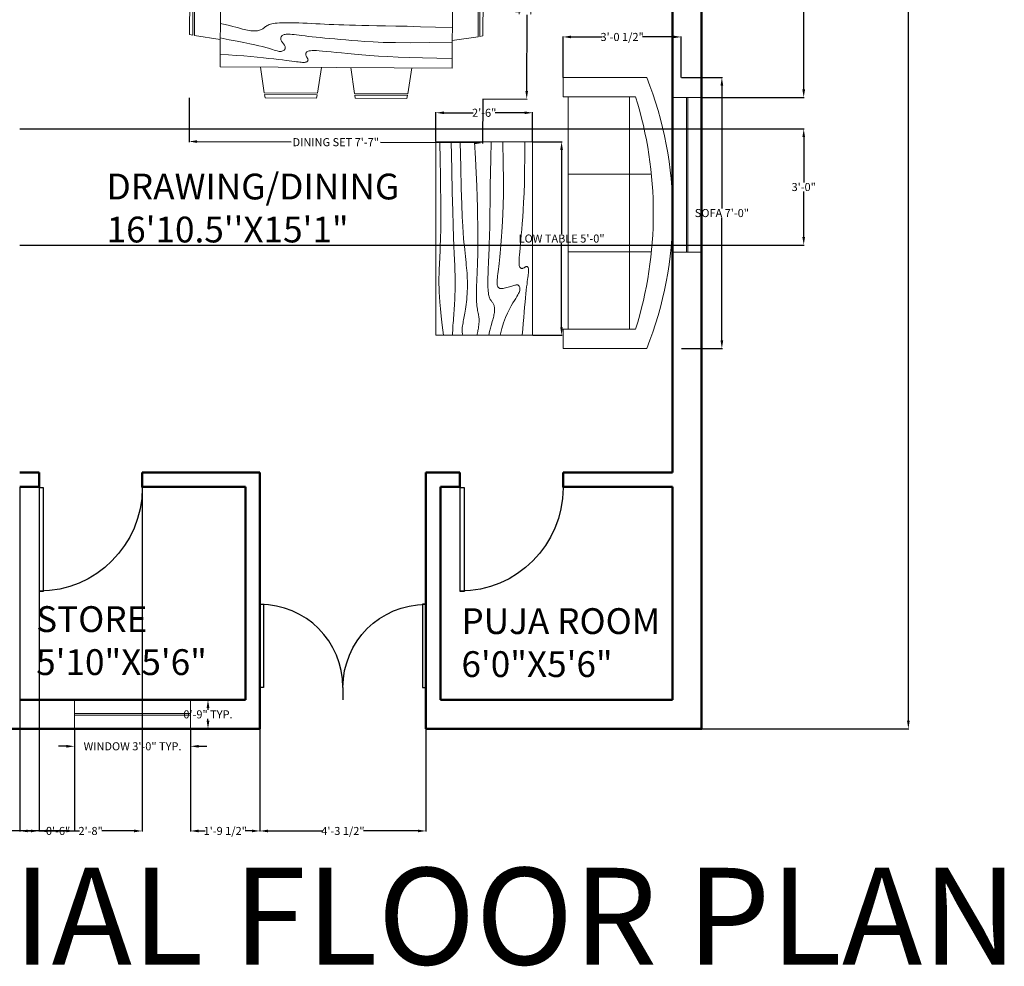
# Model space of a CAD drawing. Units: inches. Extents: x 14 to 510, y 5 to 635.
# Tile 2 of 3: x 205 to 510, y 5 to 299. Entities that reach past the tile are written whole.
import ezdxf

# ---------------------------------------------------------------- set-up
doc = ezdxf.new("R2010")
doc.units = ezdxf.units.IN
doc.header["$MEASUREMENT"] = 0
for name, color, linetype, lineweight in [('A-ANNO-DIMS', 210, 'Continuous', 18), ('A-AREA-IDEN', 210, 'Continuous', 25), ('A-FURN', 100, 'Continuous', 18), ('DOOR', 20, 'Continuous', 25), ('TEXT', 210, 'Continuous', 35), ('WALL', 40, 'Continuous', 50), ('WINDOW', 131, 'Continuous', 18)]:
    doc.layers.add(name, color=color, linetype=linetype, lineweight=lineweight)
doc.styles.get("Standard").update_dxf_attribs({"font": 'arial.ttf'})
doc.dimstyles.get("Standard").update_dxf_attribs({"dimtxt": 2.5, "dimasz": 2.5, "dimexe": 0.18, "dimexo": 0.0625, "dimgap": 0.09, "dimtad": 0, "dimtih": 1, "dimtoh": 1, "dimzin": 0, "dimdsep": 46, "dimlunit": 3, "dimtxsty": 'Standard', "dimcen": 0.09, "dimadec": 0, "dimazin": 0, "dimtfac": 1, "dimtofl": 0, "dimtmove": 0, "dimatfit": 3, "dimfxl": 1, "dimtolj": 1, "dimtzin": 0, "dimarcsym": 0})

# ---------------------------------------------------------------- blocks, each defined once
blk = doc.blocks.new('*U2')
for p, q in [((0, 0), (0, -6)), ((40, 0), (40, -6))]:
    blk.add_line(p, q)
blk.add_lwpolyline([(0, 0), (0, 40), (1.75, 40), (1.75, 0)], close=True)
blk.add_arc((0, 0), 40, 0, 90)
blk = doc.blocks.new('Dining Set - 36 x 72 in.')
for p, q in [((-22, 27.5), (-22.1562, 26.50042)), ((-22, 27.5), (-6, 27.5)), ((-5.8437, 26.49966), (-6, 27.5)), ((6, 27.5), (5.8438, 26.50042)), ((6, 27.5), (22, 27.5)), ((22.1563, 26.49966), (22, 27.5)), ((-22.2343, 26.00059), (-23.4847, 17.99762)), ((-22.2304, 26), (-5.7608, 26)), ((-5.8416, 26.5), (-22.1534, 26.5)), ((-4.5152, 17.99762), (-5.7655, 25.99926)), ((5.7657, 26.00059), (4.5153, 17.99762)), ((5.7696, 26), (22.2392, 26)), ((22.1584, 26.5), (5.8466, 26.5)), ((23.4848, 17.99762), (22.2345, 25.99926)), ((36, 18), (-36, 18)), ((-36, 18), (-36, -18)), ((36, -18), (36, 18)), ((-44.0006, 8.23428), (-35.9976, 9.48474)), ((44.0006, 8.23428), (35.9976, 9.48474)), ((-45.5, 8), (-44.5004, 8.15617)), ((-45.5, 8), (-45.5, -8)), ((-44.5, -8.15843), (-44.5, 8.15338)), ((-44, 8.23041), (-44, -8.23915)), ((44, 8.23041), (44, -8.23915)), ((44.5, -8.15843), (44.5, 8.15338)), ((45.5, 8), (44.5005, 8.15617)), ((45.5, 8), (45.5, -8)), ((-44.4997, -8.15631), (-45.5, -8)), ((-35.9976, -9.48476), (-43.9993, -8.2345)), ((35.9976, -9.48476), (43.9993, -8.2345)), ((44.4997, -8.15631), (45.5, -8)), ((-36, -18), (36, -18)), ((-22.2343, -26.0006), (-23.4847, -17.99762)), ((-4.5152, -17.99762), (-5.7655, -25.99928)), ((5.7657, -26.0006), (4.5153, -17.99762)), ((23.4848, -17.99762), (22.2345, -25.99928)), ((-22.2304, -26), (-5.7608, -26)), ((-22, -27.5), (-22.1562, -26.50044)), ((-5.8416, -26.5), (-22.1534, -26.5)), ((-5.8437, -26.49967), (-6, -27.5)), ((5.7696, -26), (22.2392, -26)), ((6, -27.5), (5.8438, -26.50044)), ((22.1584, -26.5), (5.8466, -26.5)), ((22.1563, -26.49967), (22, -27.5)), ((-22, -27.5), (-6, -27.5)), ((6, -27.5), (22, -27.5))]:
    blk.add_line(p, q)
for points in [[(-36, 15), (-31.1772, 14.97754), (-26.8079, 14.91406), (-22.8538, 14.81543), (-19.276, 14.6875), (-16.0362, 14.53613), (-13.0957, 14.36718), (-10.4159, 14.18652), (-7.9583, 14), (-5.6904, 13.81315), (-3.6035, 13.63021), (-1.6954, 13.45508), (0.0365, 13.29166), (1.5945, 13.14388), (2.9811, 13.01562), (4.1988, 12.9108), (5.25, 12.83333), (6.1393, 12.78613), (6.8802, 12.76823), (7.4883, 12.77767), (7.9792, 12.8125), (8.3685, 12.87077), (8.6719, 12.95052), (8.9049, 13.0498), (9.0833, 13.16666), (9.2205, 13.29899), (9.3216, 13.44401), (9.3895, 13.59879), (9.4271, 13.76041), (9.4373, 13.92594), (9.4232, 14.09245), (9.3875, 14.257), (9.3333, 14.41666), (9.2638, 14.56917), (9.1836, 14.71484), (9.0975, 14.85465), (9.0104, 14.98958), (8.9272, 15.1206), (8.8529, 15.2487), (8.7922, 15.37483), (8.75, 15.5), (8.7305, 15.62467), (8.7344, 15.74739), (8.7617, 15.86621), (8.8125, 15.97916), (8.8867, 16.08431), (8.9844, 16.17968), (9.1055, 16.26334), (9.25, 16.33333), (9.4189, 16.38802), (9.6172, 16.42708), (9.8506, 16.45052), (10.125, 16.45833), (10.4463, 16.45052), (10.8203, 16.42708), (11.2529, 16.38802), (11.75, 16.33333), (12.3184, 16.26318), (12.9694, 16.17838), (13.7151, 16.07991), (14.5677, 15.96875), (15.5395, 15.84586), (16.6426, 15.71224), (17.8893, 15.56884), (19.2917, 15.41666), (20.859, 15.25667), (22.5879, 15.08984), (24.4721, 14.91715), (26.5052, 14.73958), (28.6809, 14.5581), (30.9929, 14.3737), (33.4347, 14.18733), (36, 14)], [(-36, 10), (-28.9766, 10.14274), (-23.1725, 10.20442), (-18.4241, 10.19775), (-14.5677, 10.13541), (-11.4399, 10.03011), (-8.877, 9.89453), (-6.7154, 9.74137), (-4.7917, 9.58333), (-2.9698, 9.43082), (-1.2246, 9.28515), (0.4415, 9.14534), (2.026, 9.01041), (3.5266, 8.87939), (4.9408, 8.7513), (6.266, 8.62516), (7.5, 8.5), (8.6411, 8.37549), (9.6914, 8.2539), (10.6538, 8.13818), (11.5312, 8.03125), (12.3267, 7.93603), (13.043, 7.85547), (13.6831, 7.79248), (14.25, 7.75), (14.7471, 7.7303), (15.1797, 7.73307), (15.5537, 7.75732), (15.875, 7.80208), (16.1494, 7.86637), (16.3828, 7.94922), (16.5811, 8.04964), (16.75, 8.16666), (16.8944, 8.29915), (17.0143, 8.44531), (17.1089, 8.60319), (17.1771, 8.77083), (17.218, 8.94629), (17.2305, 9.1276), (17.2137, 9.31282), (17.1667, 9.5), (17.0895, 9.6875), (16.987, 9.875), (16.8649, 10.0625), (16.7292, 10.25), (16.5856, 10.4375), (16.4401, 10.625), (16.2985, 10.8125), (16.1667, 11), (16.05, 11.18733), (15.9518, 11.3737), (15.8752, 11.5581), (15.8229, 11.73958), (15.798, 11.91715), (15.8034, 12.08984), (15.842, 12.25667), (15.9167, 12.41666), (16.0295, 12.56836), (16.1784, 12.70833), (16.3605, 12.83268), (16.5729, 12.9375), (16.8127, 13.01888), (17.0768, 13.07291), (17.3625, 13.0957), (17.6667, 13.08333), (17.9894, 13.03312), (18.3418, 12.94726), (18.7382, 12.82918), (19.1927, 12.68229), (19.7195, 12.51001), (20.3327, 12.31575), (21.0465, 12.10294), (21.875, 11.875), (22.8357, 11.63354), (23.959, 11.37304), (25.2786, 11.08618), (26.8282, 10.76562), (28.6414, 10.40405), (30.752, 9.99414), (33.1936, 9.52856), (36, 9)], [(-36, 5.5), (-30.7157, 5.3348), (-26.069, 5.20963), (-21.9946, 5.11767), (-18.4271, 5.05208), (-15.3009, 5.00602), (-12.5508, 4.97265), (-10.1112, 4.94515), (-7.9167, 4.91666), (-5.909, 4.88167), (-4.0586, 4.83984), (-2.3429, 4.79215), (-0.7396, 4.73958), (0.7739, 4.6831), (2.22, 4.6237), (3.6213, 4.56233), (5, 4.5), (6.373, 4.43782), (7.7344, 4.3776), (9.0723, 4.32129), (10.375, 4.27083), (11.6309, 4.22819), (12.8281, 4.19531), (13.9551, 4.17415), (15, 4.16666), (15.954, 4.17448), (16.819, 4.19791), (17.6001, 4.23698), (18.3021, 4.29166), (18.9299, 4.36198), (19.4883, 4.44791), (19.9823, 4.54948), (20.4167, 4.66666), (20.7969, 4.79899), (21.1302, 4.94401), (21.4245, 5.09879), (21.6875, 5.26041), (21.9271, 5.42594), (22.1511, 5.59245), (22.3672, 5.757), (22.5834, 5.91666), (22.8065, 6.06868), (23.0404, 6.21093), (23.2879, 6.34147), (23.5521, 6.45833), (23.8358, 6.55957), (24.142, 6.64323), (24.4735, 6.70735), (24.8334, 6.75), (25.2235, 6.76969), (25.642, 6.76692), (26.0858, 6.74267), (26.5521, 6.69791), (27.0379, 6.63362), (27.5404, 6.55078), (28.0565, 6.45036), (28.5834, 6.33333), (29.1242, 6.19987), (29.7071, 6.04687), (30.3661, 5.87044), (31.1354, 5.66666), (32.0493, 5.43164), (33.142, 5.16146), (34.4475, 4.85221), (36, 4.5)], [(-36, -1), (-30.7915, -0.6591), (-26.0195, -0.38216), (-21.6519, -0.16284), (-17.6563, 0.00521), (-14.0005, 0.12833), (-10.6523, 0.21289), (-7.5796, 0.26522), (-4.75, 0.29166), (-2.134, 0.29793), (0.2878, 0.28711), (2.5317, 0.26163), (4.6146, 0.22396), (6.5529, 0.17651), (8.3633, 0.12174), (10.0623, 0.06209), (11.6667, 0), (13.1899, -0.06201), (14.6341, -0.1211), (15.9982, -0.17432), (17.2813, -0.21875), (18.4823, -0.25147), (19.6003, -0.26953), (20.6343, -0.27002), (21.5834, -0.25), (22.4481, -0.20768), (23.2357, -0.14584), (23.9549, -0.06836), (24.6146, 0.02083), (25.2235, 0.11784), (25.7904, 0.21875), (26.3241, 0.31966), (26.8334, 0.41666), (27.3265, 0.50618), (27.8099, 0.58593), (28.2894, 0.65397), (28.7709, 0.70833), (29.2601, 0.74707), (29.763, 0.76823), (30.2855, 0.76985), (30.8334, 0.75), (31.4088, 0.70784), (31.9994, 0.64713), (32.589, 0.57275), (33.1615, 0.48958), (33.7008, 0.4025), (34.1908, 0.3164), (34.6153, 0.23616), (34.9584, 0.16666), (35.2099, 0.11165), (35.3848, 0.07031), (35.504, 0.04069), (35.5886, 0.02083), (35.6594, 0.00879), (35.7377, 0.0026), (35.8442, 0.00032), (36, 0)], [(-36, -6.5), (-27.1843, -6.31267), (-20.084, -6.1263), (-14.469, -5.9419), (-10.1094, -5.76042), (-6.7752, -5.58285), (-4.2363, -5.41016), (-2.2629, -5.24333), (-0.625, -5.08334), (0.8708, -4.93099), (2.2715, -4.78646), (3.5872, -4.64974), (4.8281, -4.52084), (6.0046, -4.39974), (7.127, -4.28646), (8.2053, -4.18099), (9.25, -4.08334), (10.2705, -3.99382), (11.2734, -3.91407), (12.2647, -3.84603), (13.25, -3.79167), (14.2354, -3.75293), (15.2266, -3.73177), (16.2295, -3.73015), (17.25, -3.75), (18.2912, -3.79248), (19.3451, -3.85547), (20.4009, -3.93604), (21.4479, -4.03125), (22.4754, -4.13819), (23.4727, -4.25391), (24.4289, -4.37549), (25.3334, -4.5), (26.1785, -4.62492), (26.9694, -4.74935), (27.7145, -4.87281), (28.4219, -4.99479), (29.1, -5.11483), (29.7572, -5.23242), (30.4016, -5.34709), (31.0417, -5.45834), (31.6837, -5.56437), (32.3262, -5.65821), (32.9658, -5.73153), (33.599, -5.77604), (34.2224, -5.78345), (34.8327, -5.74545), (35.4264, -5.65373), (36, -5.5)], [(-36, -10), (-26.4022, -9.81299), (-18.4675, -9.62891), (-11.9839, -9.45069), (-6.7396, -9.28125), (-2.5226, -9.12354), (0.8789, -8.98047), (3.6769, -8.85498), (6.0833, -8.75), (8.2767, -8.66765), (10.3021, -8.60677), (12.1712, -8.56543), (13.8958, -8.54167), (15.4876, -8.53353), (16.9583, -8.53907), (18.3197, -8.55632), (19.5834, -8.58334), (20.7616, -8.61841), (21.8685, -8.66081), (22.9188, -8.71004), (23.9271, -8.76563), (24.9081, -8.82707), (25.8763, -8.89388), (26.8465, -8.96558), (27.8334, -9.04167), (28.8474, -9.12118), (29.8828, -9.20117), (30.93, -9.27824), (31.9792, -9.34896), (33.0205, -9.40991), (34.0443, -9.45768), (35.0407, -9.48885), (36, -9.5)], [(-36, -14.5), (-30.0881, -14.33513), (-25.0332, -14.21224), (-20.7312, -14.12647), (-17.0781, -14.07292), (-13.97, -14.04671), (-11.3027, -14.04297), (-8.9724, -14.05681), (-6.875, -14.08334), (-4.9224, -14.11833), (-3.0905, -14.16016), (-1.3709, -14.20785), (0.2448, -14.26042), (1.7647, -14.3169), (3.1973, -14.3763), (4.5507, -14.43767), (5.8333, -14.5), (7.0554, -14.5621), (8.235, -14.62175), (9.3922, -14.67652), (10.5469, -14.72396), (11.7192, -14.76164), (12.929, -14.78711), (14.1965, -14.79794), (15.5417, -14.79167), (16.9933, -14.76424), (18.6152, -14.70508), (20.4804, -14.60197), (22.6615, -14.44271), (25.2312, -14.21509), (28.2624, -13.9069), (31.8277, -13.50594), (36, -13)]]:
    blk.add_lwpolyline(points)
blk = doc.blocks.new('Table - Rectangular Woodgrain 60 x 30 in.')
for p, q in [((0, 0), (0, -30)), ((60, 0), (0, 0)), ((60, -30), (60, 0)), ((0, -30), (60, -30))]:
    blk.add_line(p, q)
for points in [[(0, -2.4), (4.8155, -2.418), (9.0302, -2.4688), (12.709, -2.5477), (15.9167, -2.65), (18.7181, -2.7711), (21.1781, -2.9063), (23.3616, -3.0508), (25.3333, -3.2), (27.1477, -3.3495), (28.8172, -3.4958), (30.3437, -3.636), (31.7291, -3.7667), (32.9756, -3.8849), (34.0849, -3.9875), (35.059, -4.0714), (35.9, -4.1334), (36.6114, -4.1711), (37.2041, -4.1854), (37.6906, -4.1779), (38.0833, -4.15), (38.3948, -4.1034), (38.6375, -4.0396), (38.8239, -3.9602), (38.9666, -3.8667), (39.0764, -3.7608), (39.1573, -3.6448), (39.2116, -3.521), (39.2416, -3.3917), (39.2498, -3.2593), (39.2385, -3.1261), (39.21, -2.9944), (39.1666, -2.8667), (39.111, -2.7447), (39.0468, -2.6281), (38.978, -2.5163), (38.9083, -2.4083), (38.8418, -2.3035), (38.7823, -2.201), (38.7337, -2.1001), (38.7, -2), (38.6844, -1.9003), (38.6875, -1.8021), (38.7094, -1.707), (38.75, -1.6167), (38.8094, -1.5326), (38.8875, -1.4563), (38.9844, -1.3893), (39.1, -1.3333), (39.2351, -1.2896), (39.3937, -1.2583), (39.5804, -1.2396), (39.8, -1.2333), (40.057, -1.2396), (40.3562, -1.2583), (40.7023, -1.2896), (41.1, -1.3333), (41.5547, -1.3895), (42.0755, -1.4573), (42.6721, -1.5361), (43.3542, -1.625), (44.1316, -1.7233), (45.014, -1.8302), (46.0114, -1.9449), (47.1333, -2.0667), (48.3862, -2.1947), (49.7625, -2.3281), (51.2513, -2.4663), (52.8416, -2.6083), (54.5226, -2.7535), (56.2833, -2.9011), (58.1127, -3.0501), (60, -3.2)], [(0, -9.2), (6.5759, -9.0858), (11.9385, -9.0365), (16.2527, -9.0418), (19.6833, -9.0917), (22.3952, -9.1759), (24.5531, -9.2844), (26.322, -9.4069), (27.8666, -9.5333), (29.3241, -9.6553), (30.7203, -9.7719), (32.0532, -9.8837), (33.3208, -9.9917), (34.5213, -10.0965), (35.6526, -10.199), (36.7128, -10.2999), (37.7, -10.4), (38.6129, -10.4996), (39.4531, -10.5969), (40.223, -10.6895), (40.925, -10.775), (41.5613, -10.8512), (42.1344, -10.9156), (42.6465, -10.966), (43.1, -11), (43.4976, -11.0158), (43.8437, -11.0136), (44.143, -10.9942), (44.4, -10.9583), (44.6195, -10.9069), (44.8062, -10.8406), (44.9648, -10.7603), (45.1, -10.6667), (45.2155, -10.5598), (45.3114, -10.4365), (45.3871, -10.2929), (45.4416, -10.125), (45.4743, -9.929), (45.4844, -9.7011), (45.4709, -9.4371), (45.4333, -9.1333), (45.3716, -8.7883), (45.2896, -8.4104), (45.1919, -8.0107), (45.0833, -7.6), (44.9685, -7.1893), (44.8521, -6.7896), (44.7388, -6.4117), (44.6333, -6.0667), (44.54, -5.7628), (44.4614, -5.4979), (44.4001, -5.2675), (44.3583, -5.0667), (44.3384, -4.8909), (44.3427, -4.7354), (44.3736, -4.5956), (44.4333, -4.4667), (44.5236, -4.3453), (44.6427, -4.2333), (44.7884, -4.1339), (44.9583, -4.05), (45.1501, -3.9849), (45.3614, -3.9417), (45.59, -3.9234), (45.8333, -3.9333), (46.0915, -3.9749), (46.3734, -4.0531), (46.6906, -4.1736), (47.0542, -4.3417), (47.4756, -4.5629), (47.9661, -4.8427), (48.5372, -5.1866), (49.2, -5.6), (49.9676, -6.0844), (50.8594, -6.625), (51.8965, -7.2031), (53.1, -7.8), (54.491, -8.3969), (56.0906, -8.975), (57.9199, -9.5156), (60, -10)], [(0, -12.8), (5.1847, -12.9322), (9.6213, -13.0323), (13.3963, -13.1059), (16.5958, -13.1583), (19.3063, -13.1952), (21.614, -13.2219), (23.6054, -13.2439), (25.3666, -13.2667), (26.9728, -13.2947), (28.4531, -13.3281), (29.8256, -13.3663), (31.1083, -13.4083), (32.3191, -13.4535), (33.476, -13.501), (34.597, -13.5501), (35.7, -13.6), (36.7984, -13.6497), (37.8875, -13.6979), (38.9578, -13.743), (40, -13.7833), (41.0047, -13.8174), (41.9625, -13.8438), (42.864, -13.8607), (43.7, -13.8667), (44.4631, -13.8604), (45.1552, -13.8417), (45.7801, -13.8104), (46.3416, -13.7667), (46.8439, -13.7104), (47.2906, -13.6417), (47.6858, -13.5604), (48.0333, -13.4667), (48.3375, -13.3608), (48.6042, -13.2448), (48.8396, -13.121), (49.05, -12.9917), (49.2417, -12.8593), (49.4208, -12.7261), (49.5937, -12.5944), (49.7667, -12.4667), (49.9452, -12.3451), (50.1323, -12.2313), (50.3303, -12.1268), (50.5416, -12.0333), (50.7686, -11.9524), (51.0135, -11.8854), (51.2788, -11.8341), (51.5666, -11.8), (51.8785, -11.7843), (52.2116, -11.7865), (52.562, -11.8059), (52.926, -11.8417), (53.2998, -11.8931), (53.6795, -11.9594), (54.0614, -12.0397), (54.4416, -12.1333), (54.8223, -12.2401), (55.2293, -12.3625), (55.6942, -12.5037), (56.2489, -12.6667), (56.9251, -12.8547), (57.7545, -13.0708), (58.7689, -13.3182), (60, -13.6)], [(0, -18), (5.124, -17.7273), (9.6609, -17.5057), (13.6705, -17.3303), (17.2125, -17.1958), (20.3467, -17.0973), (23.1328, -17.0297), (25.6307, -16.9878), (27.9, -16.9667), (29.9928, -16.9617), (31.9302, -16.9703), (33.7254, -16.9907), (35.3917, -17.0208), (36.9423, -17.0588), (38.3906, -17.1026), (39.7499, -17.1503), (41.0333, -17.2), (42.2519, -17.2496), (43.4073, -17.2969), (44.4986, -17.3395), (45.525, -17.375), (46.4858, -17.4012), (47.3802, -17.4156), (48.2074, -17.416), (48.9667, -17.4), (49.6583, -17.3662), (50.2872, -17.3167), (50.8595, -17.2547), (51.3812, -17.1833), (51.8584, -17.1057), (52.2971, -17.025), (52.7034, -16.9443), (53.0833, -16.8667), (53.443, -16.7951), (53.789, -16.7313), (54.128, -16.6768), (54.4666, -16.6334), (54.8115, -16.6024), (55.1693, -16.5854), (55.5465, -16.5841), (55.95, -16.6), (56.3828, -16.6337), (56.8346, -16.6823), (57.2915, -16.7418), (57.7396, -16.8084), (58.165, -16.878), (58.5539, -16.9469), (58.8924, -17.0111), (59.1666, -17.0667), (59.3679, -17.1107), (59.5078, -17.1438), (59.6032, -17.1675), (59.6708, -17.1833), (59.7275, -17.193), (59.7901, -17.1979), (59.8753, -17.1998), (60, -17.2)], [(0, -22.4), (8.0098, -22.2501), (14.4094, -22.1011), (19.4168, -21.9535), (23.25, -21.8083), (26.1269, -21.6663), (28.2656, -21.5281), (29.884, -21.3947), (31.2, -21.2667), (32.3967, -21.1448), (33.5172, -21.0292), (34.5697, -20.9198), (35.5625, -20.8167), (36.5037, -20.7198), (37.4015, -20.6292), (38.2642, -20.5448), (39.1, -20.4667), (39.9164, -20.3951), (40.7187, -20.3313), (41.5117, -20.2768), (42.3, -20.2333), (43.0883, -20.2024), (43.8812, -20.1854), (44.6836, -20.1841), (45.5, -20.2), (46.3328, -20.234), (47.1747, -20.2844), (48.0163, -20.3488), (48.8479, -20.425), (49.66, -20.5106), (50.4429, -20.6031), (51.1872, -20.7004), (51.8833, -20.8), (52.5246, -20.8999), (53.1166, -20.9995), (53.6681, -21.0983), (54.1875, -21.1958), (54.6834, -21.2919), (55.1646, -21.3859), (55.6394, -21.4777), (56.1167, -21.5667), (56.6028, -21.6515), (57.0961, -21.7266), (57.5929, -21.7852), (58.0896, -21.8208), (58.5823, -21.8268), (59.0674, -21.7964), (59.5412, -21.723), (60, -21.6)], [(0, -25.2), (8.6355, -25.0504), (15.7026, -24.9031), (21.4049, -24.7606), (25.9458, -24.625), (29.529, -24.4988), (32.3578, -24.3844), (34.6359, -24.284), (36.5667, -24.2), (38.3213, -24.1341), (39.9417, -24.0854), (41.437, -24.0523), (42.8167, -24.0333), (44.0901, -24.0268), (45.2667, -24.0313), (46.3557, -24.0451), (47.3667, -24.0667), (48.309, -24.0947), (49.1928, -24.1287), (50.0284, -24.168), (50.826, -24.2125), (51.5959, -24.2617), (52.3483, -24.3151), (53.0935, -24.3725), (53.8417, -24.4334), (54.6009, -24.497), (55.3699, -24.561), (56.1454, -24.6226), (56.9239, -24.6792), (57.7021, -24.7279), (58.4764, -24.7662), (59.2435, -24.7911), (60, -24.8)], [(0, -28.8), (5.6867, -28.6681), (10.45, -28.5698), (14.407, -28.5012), (17.675, -28.4584), (20.3711, -28.4374), (22.6125, -28.4344), (24.5164, -28.4455), (26.2, -28.4667), (27.762, -28.4947), (29.2276, -28.5281), (30.6033, -28.5663), (31.8958, -28.6084), (33.1118, -28.6535), (34.2578, -28.7011), (35.3405, -28.7501), (36.3666, -28.8), (37.3443, -28.8497), (38.288, -28.8974), (39.2137, -28.9412), (40.1375, -28.9792), (41.0753, -29.0093), (42.0432, -29.0297), (43.0572, -29.0384), (44.1333, -29.0333), (45.2936, -29.0114), (46.5843, -28.9641), (48.0579, -28.8816), (49.7666, -28.7542), (51.7629, -28.5721), (54.0989, -28.3255), (56.8272, -28.0048), (60, -27.6)]]:
    blk.add_lwpolyline(points)
blk = doc.blocks.new('Sofa - Roundback 7 ft.')
for p, q in [((-12.00002, -32.4421), (-12.00003, -6.5971)), ((11.99997, -32.4421), (11.99998, -6.5971)), ((-36.000027, -34), (-36.000027, -11.4696)), ((35.99998, -34), (35.99998, -11.4696)), ((-35.999844, -13.3819), (35.9998, -13.3819)), ((-36.000027, -32.4421), (35.99998, -32.4421))]:
    blk.add_line(p, q)
for points in [[(-36.000027, -34), (-42.000027, -34), (-42.000027, -8)], [(41.99998, -8), (41.99998, -34), (35.99998, -34)]]:
    blk.add_lwpolyline(points)
for centre, radius, start, end in [((0, -114.25), 114.25, 68.43141, 111.5686), ((-0.00001, -127.1968), 121.1968, 72.72033, 107.2797)]:
    blk.add_arc(centre, radius, start, end)
blk = doc.blocks.new('*D14')
at = {"layer": 'A-ANNO-DIMS', "color": 0, "lineweight": -2, "transparency": 16777216}
for p, q in [((416.67, 559.06), (480.9, 559.06)), ((480.72, 556.56), (480.72, 325.28)), ((480.72, 81.56), (480.72, 312.84)), ((416.67, 79.06), (480.9, 79.06))]:
    blk.add_line(p, q, dxfattribs=at)
at = {"layer": 'A-ANNO-DIMS', "color": 0, "transparency": 16777216}
for points in [[(480.3, 556.56), (481.13, 556.56), (480.72, 559.06)], [(480.3, 81.56), (481.13, 81.56), (480.72, 79.06)]]:
    blk.add_solid(points, dxfattribs=at)
at = {"layer": 'Defpoints', "color": 0, "transparency": 16777216}
for p in [(416.61, 559.06), (416.61, 79.06), (480.72, 79.06)]:
    blk.add_point(p, dxfattribs=at)
at = {"layer": 'A-ANNO-DIMS', "color": 0, "transparency": 16777216, "insert": (480.72, 319.06), "char_height": 12, "attachment_point": 5}
blk.add_mtext("\\A1;40'", dxfattribs=at)
blk = doc.blocks.new('WIN-48IN')
for p, q in [((4.25, 48), (4.25, 0)), ((4.75, 48), (4.75, 0))]:
    blk.add_line(p, q)
blk.add_lwpolyline([(0, 48), (0, 0), (9, 0), (9, 48)], close=True)
blk = doc.blocks.new('WIN-36IN')
for p, q in [((0, 4.75), (36, 4.75)), ((0, 4.25), (36, 4.25))]:
    blk.add_line(p, q)
blk.add_lwpolyline([(0, 0), (36, 0), (36, 9), (0, 9)], close=True)
blk = doc.blocks.new('*D21')
at = {"layer": 'A-ANNO-DIMS', "color": 0, "lineweight": -2, "transparency": 16777216}
for p, q in [((222.11, 79), (222.11, 73.48)), ((258.11, 79), (258.11, 73.48)), ((219.61, 73.66), (217.11, 73.66)), ((260.61, 73.66), (263.11, 73.66))]:
    blk.add_line(p, q, dxfattribs=at)
at = {"layer": 'A-ANNO-DIMS', "color": 0, "transparency": 16777216}
for points in [[(219.61, 74.08), (219.61, 73.24), (222.11, 73.66)], [(260.61, 74.08), (260.61, 73.24), (258.11, 73.66)]]:
    blk.add_solid(points, dxfattribs=at)
at = {"layer": 'Defpoints', "color": 0, "transparency": 16777216}
for p in [(222.11, 79.06), (258.11, 79.06), (258.11, 73.66)]:
    blk.add_point(p, dxfattribs=at)
at = {"layer": 'A-ANNO-DIMS', "color": 0, "transparency": 16777216, "insert": (240.11, 73.66), "char_height": 2.5, "attachment_point": 5}
blk.add_mtext('\\A1;WINDOW 3\'-0" TYP.', dxfattribs=at)
blk = doc.blocks.new('*D22')
at = {"layer": 'A-ANNO-DIMS', "color": 0, "lineweight": -2, "transparency": 16777216}
for p, q in [((258.17, 88.06), (263.69, 88.06)), ((263.51, 85.56), (263.51, 84.93)), ((263.51, 81.56), (263.51, 82.19)), ((258.17, 79.06), (263.69, 79.06))]:
    blk.add_line(p, q, dxfattribs=at)
at = {"layer": 'A-ANNO-DIMS', "color": 0, "transparency": 16777216}
for points in [[(263.09, 85.56), (263.93, 85.56), (263.51, 88.06)], [(263.09, 81.56), (263.93, 81.56), (263.51, 79.06)]]:
    blk.add_solid(points, dxfattribs=at)
at = {"layer": 'Defpoints', "color": 0, "transparency": 16777216}
for p in [(258.11, 88.06), (263.51, 88.06), (258.11, 79.06)]:
    blk.add_point(p, dxfattribs=at)
at = {"layer": 'A-ANNO-DIMS', "color": 0, "transparency": 16777216, "insert": (263.51, 83.56), "char_height": 2.5, "attachment_point": 5}
blk.add_mtext('\\A1;0\'-9" TYP.', dxfattribs=at)
blk = doc.blocks.new('*D29')
at = {"layer": 'A-ANNO-DIMS', "color": 0, "lineweight": -2, "transparency": 16777216}
for p, q in [((257.7, 274.76), (257.64, 260.99)), ((348.7, 274.33), (348.63, 260.56)), ((260.14, 261.16), (289.31, 261.02)), ((346.14, 260.75), (316.97, 260.89))]:
    blk.add_line(p, q, dxfattribs=at)
at = {"layer": 'A-ANNO-DIMS', "color": 0, "transparency": 16777216}
for points in [[(260.14, 261.58), (260.13, 260.74), (257.64, 261.17)], [(346.14, 261.17), (346.13, 260.34), (348.64, 260.74)]]:
    blk.add_solid(points, dxfattribs=at)
at = {"layer": 'Defpoints', "color": 0, "transparency": 16777216}
for p in [(257.7, 274.82), (348.7, 274.39), (257.64, 261.17)]:
    blk.add_point(p, dxfattribs=at)
at = {"layer": 'A-ANNO-DIMS', "color": 0, "transparency": 16777216, "insert": (303.14, 260.96), "char_height": 2.5, "attachment_point": 5}
blk.add_mtext('\\A1;DINING SET 7\'-7"', dxfattribs=at)
blk = doc.blocks.new('*D30')
at = {"layer": 'A-ANNO-DIMS', "color": 0, "lineweight": -2, "transparency": 16777216}
for p, q in [((349.02, 329.39), (362.79, 329.33)), ((362.6, 326.83), (362.49, 303.17)), ((362.36, 276.83), (362.47, 300.49)), ((348.76, 274.39), (362.53, 274.33))]:
    blk.add_line(p, q, dxfattribs=at)
at = {"layer": 'A-ANNO-DIMS', "color": 0, "transparency": 16777216}
for points in [[(362.18, 326.83), (363.02, 326.82), (362.61, 329.33)], [(361.95, 276.83), (362.78, 276.83), (362.35, 274.33)]]:
    blk.add_solid(points, dxfattribs=at)
at = {"layer": 'Defpoints', "color": 0, "transparency": 16777216}
for p in [(348.96, 329.39), (348.7, 274.39), (362.35, 274.33)]:
    blk.add_point(p, dxfattribs=at)
at = {"layer": 'A-ANNO-DIMS', "color": 0, "transparency": 16777216, "insert": (362.48, 301.83), "char_height": 2.5, "attachment_point": 5}
blk.add_mtext('\\A1;4\'-7"', dxfattribs=at)
blk = doc.blocks.new('*D31')
at = {"layer": 'A-ANNO-DIMS', "color": 0, "lineweight": -2, "transparency": 16777216}
for p, q in [((364.23, 261.08), (373.35, 261.08)), ((373.17, 258.58), (373.17, 232.46)), ((373.17, 203.58), (373.17, 229.69)), ((364.23, 201.08), (373.35, 201.08))]:
    blk.add_line(p, q, dxfattribs=at)
at = {"layer": 'A-ANNO-DIMS', "color": 0, "transparency": 16777216}
for points in [[(372.75, 258.58), (373.58, 258.58), (373.17, 261.08)], [(372.75, 203.58), (373.58, 203.58), (373.17, 201.08)]]:
    blk.add_solid(points, dxfattribs=at)
at = {"layer": 'Defpoints', "color": 0, "transparency": 16777216}
for p in [(364.17, 261.08), (364.17, 201.08), (373.17, 201.08)]:
    blk.add_point(p, dxfattribs=at)
at = {"layer": 'A-ANNO-DIMS', "color": 0, "transparency": 16777216, "insert": (373.17, 231.08), "char_height": 2.5, "attachment_point": 5}
blk.add_mtext('\\A1;LOW TABLE 5\'-0"', dxfattribs=at)
blk = doc.blocks.new('*D32')
at = {"layer": 'A-ANNO-DIMS', "color": 0, "lineweight": -2, "transparency": 16777216}
for p, q in [((334.17, 261.14), (334.17, 270.26)), ((336.67, 270.08), (345.73, 270.08)), ((361.67, 270.08), (352.6, 270.08)), ((364.17, 261.14), (364.17, 270.26))]:
    blk.add_line(p, q, dxfattribs=at)
at = {"layer": 'A-ANNO-DIMS', "color": 0, "transparency": 16777216}
for points in [[(336.67, 270.49), (336.67, 269.66), (334.17, 270.08)], [(361.67, 270.49), (361.67, 269.66), (364.17, 270.08)]]:
    blk.add_solid(points, dxfattribs=at)
at = {"layer": 'Defpoints', "color": 0, "transparency": 16777216}
for p in [(364.17, 270.08), (334.17, 261.08), (364.17, 261.08)]:
    blk.add_point(p, dxfattribs=at)
at = {"layer": 'A-ANNO-DIMS', "color": 0, "transparency": 16777216, "insert": (349.17, 270.08), "char_height": 2.5, "attachment_point": 5}
blk.add_mtext('\\A1;2\'-6"', dxfattribs=at)
blk = doc.blocks.new('*D33')
at = {"layer": 'A-ANNO-DIMS', "color": 0, "lineweight": -2, "transparency": 16777216}
for p, q in [((410.34, 280.99), (423.06, 280.99)), ((422.88, 278.49), (422.88, 240.38)), ((422.88, 199.49), (422.88, 237.61)), ((410.34, 196.99), (423.06, 196.99))]:
    blk.add_line(p, q, dxfattribs=at)
at = {"layer": 'A-ANNO-DIMS', "color": 0, "transparency": 16777216}
for points in [[(422.46, 278.49), (423.29, 278.49), (422.88, 280.99)], [(422.46, 199.49), (423.29, 199.49), (422.88, 196.99)]]:
    blk.add_solid(points, dxfattribs=at)
at = {"layer": 'Defpoints', "color": 0, "transparency": 16777216}
for p in [(410.28, 280.99), (410.28, 196.99), (422.88, 196.99)]:
    blk.add_point(p, dxfattribs=at)
at = {"layer": 'A-ANNO-DIMS', "color": 0, "transparency": 16777216, "insert": (422.88, 238.99), "char_height": 2.5, "attachment_point": 5}
blk.add_mtext('\\A1;SOFA 7\'-0"', dxfattribs=at)
blk = doc.blocks.new('*D34')
at = {"layer": 'A-ANNO-DIMS', "color": 0, "lineweight": -2, "transparency": 16777216}
for p, q in [((373.61, 281.06), (373.61, 293.77)), ((376.11, 293.59), (385.62, 293.59)), ((407.78, 293.59), (398.27, 293.59)), ((410.28, 281.06), (410.28, 293.77))]:
    blk.add_line(p, q, dxfattribs=at)
at = {"layer": 'A-ANNO-DIMS', "color": 0, "transparency": 16777216}
for points in [[(376.11, 294.01), (376.11, 293.18), (373.61, 293.59)], [(407.78, 294.01), (407.78, 293.18), (410.28, 293.59)]]:
    blk.add_solid(points, dxfattribs=at)
at = {"layer": 'Defpoints', "color": 0, "transparency": 16777216}
for p in [(410.28, 293.59), (373.61, 280.99), (410.28, 280.99)]:
    blk.add_point(p, dxfattribs=at)
at = {"layer": 'A-ANNO-DIMS', "color": 0, "transparency": 16777216, "insert": (391.94, 293.59), "char_height": 2.5, "attachment_point": 5}
blk.add_mtext('\\A1;3\'-0 1/2"', dxfattribs=at)
blk = doc.blocks.new('*D43')
at = {"layer": 'A-ANNO-DIMS', "color": 0, "lineweight": -2, "transparency": 16777216}
for p, q in [((151.11, 79), (151.11, 47.23)), ((222.11, 79), (222.11, 47.23)), ((153.61, 47.41), (182.23, 47.41)), ((219.61, 47.41), (190.99, 47.41))]:
    blk.add_line(p, q, dxfattribs=at)
at = {"layer": 'A-ANNO-DIMS', "color": 0, "transparency": 16777216}
for points in [[(153.61, 47.83), (153.61, 46.99), (151.11, 47.41)], [(219.61, 47.83), (219.61, 46.99), (222.11, 47.41)]]:
    blk.add_solid(points, dxfattribs=at)
at = {"layer": 'Defpoints', "color": 0, "transparency": 16777216}
for p in [(151.11, 79.06), (222.11, 79.06), (222.11, 47.41)]:
    blk.add_point(p, dxfattribs=at)
at = {"layer": 'A-ANNO-DIMS', "color": 0, "transparency": 16777216, "insert": (186.61, 47.41), "char_height": 2.5, "attachment_point": 5}
blk.add_mtext('\\A1;5\'-11"', dxfattribs=at)
blk = doc.blocks.new('*D44')
at = {"layer": 'A-ANNO-DIMS', "color": 0, "lineweight": -2, "transparency": 16777216}
for p, q in [((258.11, 79), (258.11, 47.23)), ((279.61, 79), (279.61, 47.23)), ((260.61, 47.41), (262.65, 47.41)), ((277.11, 47.41), (275.07, 47.41))]:
    blk.add_line(p, q, dxfattribs=at)
at = {"layer": 'A-ANNO-DIMS', "color": 0, "transparency": 16777216}
for points in [[(260.61, 47.83), (260.61, 46.99), (258.11, 47.41)], [(277.11, 47.83), (277.11, 46.99), (279.61, 47.41)]]:
    blk.add_solid(points, dxfattribs=at)
at = {"layer": 'Defpoints', "color": 0, "transparency": 16777216}
for p in [(258.11, 79.06), (279.61, 79.06), (279.61, 47.41)]:
    blk.add_point(p, dxfattribs=at)
at = {"layer": 'A-ANNO-DIMS', "color": 0, "transparency": 16777216, "insert": (268.86, 47.41), "char_height": 2.5, "attachment_point": 5}
blk.add_mtext('\\A1;1\'-9 1/2"', dxfattribs=at)
blk = doc.blocks.new('*D45')
at = {"layer": 'A-ANNO-DIMS', "color": 0, "lineweight": -2, "transparency": 16777216}
for p, q in [((279.61, 79), (279.61, 47.23)), ((331.11, 79), (331.11, 47.23)), ((282.11, 47.41), (298.99, 47.41)), ((328.61, 47.41), (311.74, 47.41))]:
    blk.add_line(p, q, dxfattribs=at)
at = {"layer": 'A-ANNO-DIMS', "color": 0, "transparency": 16777216}
for points in [[(282.11, 47.83), (282.11, 46.99), (279.61, 47.41)], [(328.61, 47.83), (328.61, 46.99), (331.11, 47.41)]]:
    blk.add_solid(points, dxfattribs=at)
at = {"layer": 'Defpoints', "color": 0, "transparency": 16777216}
for p in [(279.61, 79.06), (331.11, 79.06), (331.11, 47.41)]:
    blk.add_point(p, dxfattribs=at)
at = {"layer": 'A-ANNO-DIMS', "color": 0, "transparency": 16777216, "insert": (305.36, 47.41), "char_height": 2.5, "attachment_point": 5}
blk.add_mtext('\\A1;4\'-3 1/2"', dxfattribs=at)
blk = doc.blocks.new('*D49')
at = {"layer": 'A-ANNO-DIMS', "color": 0, "lineweight": -2, "transparency": 16777216}
for p, q in [((416.67, 395.56), (448.44, 395.56)), ((448.26, 393.06), (448.26, 336.55)), ((448.26, 277.31), (448.26, 333.82)), ((416.67, 274.81), (448.44, 274.81))]:
    blk.add_line(p, q, dxfattribs=at)
at = {"layer": 'A-ANNO-DIMS', "color": 0, "transparency": 16777216}
for points in [[(447.84, 393.06), (448.68, 393.06), (448.26, 395.56)], [(447.84, 277.31), (448.68, 277.31), (448.26, 274.81)]]:
    blk.add_solid(points, dxfattribs=at)
at = {"layer": 'Defpoints', "color": 0, "transparency": 16777216}
for p in [(416.61, 395.56), (416.61, 274.81), (448.26, 274.81)]:
    blk.add_point(p, dxfattribs=at)
at = {"layer": 'A-ANNO-DIMS', "color": 0, "transparency": 16777216, "insert": (448.26, 335.19), "char_height": 2.5, "attachment_point": 5}
blk.add_mtext('\\A1;10\'-1"', dxfattribs=at)
blk = doc.blocks.new('*D50')
at = {"layer": 'A-ANNO-DIMS', "color": 0, "lineweight": -2, "transparency": 16777216}
for p, q in [((205.17, 265.06), (448.44, 265.06)), ((448.26, 262.56), (448.26, 248.43)), ((448.26, 231.56), (448.26, 245.69)), ((205.17, 229.06), (448.44, 229.06))]:
    blk.add_line(p, q, dxfattribs=at)
at = {"layer": 'A-ANNO-DIMS', "color": 0, "transparency": 16777216}
for points in [[(447.84, 262.56), (448.68, 262.56), (448.26, 265.06)], [(447.84, 231.56), (448.68, 231.56), (448.26, 229.06)]]:
    blk.add_solid(points, dxfattribs=at)
at = {"layer": 'Defpoints', "color": 0, "transparency": 16777216}
for p in [(205.11, 265.06), (448.26, 265.06), (205.11, 229.06)]:
    blk.add_point(p, dxfattribs=at)
at = {"layer": 'A-ANNO-DIMS', "color": 0, "transparency": 16777216, "insert": (448.26, 247.06), "char_height": 2.5, "attachment_point": 5}
blk.add_mtext('\\A1;3\'-0"', dxfattribs=at)
blk = doc.blocks.new('*D53')
at = {"layer": 'A-ANNO-DIMS', "color": 0, "lineweight": -2, "transparency": 16777216}
for p, q in [((205.11, 154), (205.11, 47.23)), ((211.11, 154), (211.11, 47.23)), ((207.61, 47.41), (208.61, 47.41)), ((211.11, 47.41), (213.61, 47.41))]:
    blk.add_line(p, q, dxfattribs=at)
at = {"layer": 'A-ANNO-DIMS', "color": 0, "transparency": 16777216}
for points in [[(207.61, 47.83), (207.61, 46.99), (205.11, 47.41)], [(208.61, 47.83), (208.61, 46.99), (211.11, 47.41)]]:
    blk.add_solid(points, dxfattribs=at)
at = {"layer": 'Defpoints', "color": 0, "transparency": 16777216}
for p in [(205.11, 154.06), (211.11, 154.06), (211.11, 47.41)]:
    blk.add_point(p, dxfattribs=at)
at = {"layer": 'A-ANNO-DIMS', "color": 0, "transparency": 16777216, "insert": (217.02, 47.41), "char_height": 2.5, "attachment_point": 5}
blk.add_mtext('\\A1;0\'-6"', dxfattribs=at)
blk = doc.blocks.new('*D54')
at = {"layer": 'A-ANNO-DIMS', "color": 0, "lineweight": -2, "transparency": 16777216}
for p, q in [((211.11, 154), (211.11, 47.23)), ((243.11, 154), (243.11, 47.23)), ((213.61, 47.41), (223.68, 47.41)), ((240.61, 47.41), (230.55, 47.41))]:
    blk.add_line(p, q, dxfattribs=at)
at = {"layer": 'A-ANNO-DIMS', "color": 0, "transparency": 16777216}
for points in [[(213.61, 47.83), (213.61, 46.99), (211.11, 47.41)], [(240.61, 47.83), (240.61, 46.99), (243.11, 47.41)]]:
    blk.add_solid(points, dxfattribs=at)
at = {"layer": 'Defpoints', "color": 0, "transparency": 16777216}
for p in [(211.11, 154.06), (243.11, 154.06), (243.11, 47.41)]:
    blk.add_point(p, dxfattribs=at)
at = {"layer": 'A-ANNO-DIMS', "color": 0, "transparency": 16777216, "insert": (227.11, 47.41), "char_height": 2.5, "attachment_point": 5}
blk.add_mtext('\\A1;2\'-8"', dxfattribs=at)

msp = doc.modelspace()

# ---------------------------------------------------------------- linework, layer by layer
at = {"layer": 'WALL'}
for p, q in [((407.611, 158.561), (407.611, 343.061)), ((205.111, 158.561), (211.111, 158.561)), ((211.111, 158.561), (211.111, 154.061)), ((243.111, 158.561), (243.111, 154.061)), ((243.111, 158.561), (279.611, 158.561)), ((279.611, 158.561), (279.611, 88.061)), ((331.111, 88.061), (331.111, 158.561)), ((331.111, 158.561), (341.611, 158.561)), ((341.611, 154.061), (341.611, 158.561)), ((373.611, 154.061), (373.611, 158.561)), ((373.611, 158.561), (407.611, 158.561)), ((205.111, 154.061), (211.111, 154.061)), ((243.111, 154.061), (275.111, 154.061)), ((275.111, 154.061), (275.111, 88.061)), ((335.611, 88.061), (335.611, 154.061)), ((335.611, 154.061), (341.611, 154.061)), ((373.611, 154.061), (407.611, 154.061)), ((407.611, 88.061), (407.611, 154.061)), ((205.111, 88.061), (275.111, 88.061)), ((279.611, 88.061), (279.611, 79.061)), ((331.111, 88.061), (331.111, 79.061)), ((335.611, 88.061), (407.611, 88.061))]:
    msp.add_line(p, q, dxfattribs=at)
msp.add_lwpolyline([(331.111, 79.061), (416.611, 79.061), (416.611, 559.061), (56.611, 559.061), (56.611, 79.061), (279.611, 79.061)], dxfattribs=at)

# ---------------------------------------------------------------- block references
at = {"layer": 'A-FURN'}
for name, p, rotation in [('Dining Set - 36 x 72 in.', (303.331, 302.107), 179.7284420558059), ('Sofa - Roundback 7 ft.', (407.611, 238.993), 270), ('Table - Rectangular Woodgrain 60 x 30 in.', (364.167, 261.076), 270)]:
    msp.add_blockref(name, p, dxfattribs=dict(at, rotation=rotation))
at = {"layer": 'DOOR', "rotation": 180}
for p, xscale, yscale, zscale in [((211.111, 153.761), -0.7999999999999994, 0.7999999999999994, 0.7999999999999994), ((341.611, 153.761), -0.7999999999999998, 0.7999999999999998, 0.7999999999999998)]:
    msp.add_blockref('*U2', p, dxfattribs=dict(at, xscale=xscale, yscale=yscale, zscale=zscale))
at = {"layer": 'DOOR', "yscale": 0.6437500000000015, "zscale": 0.6437500000000015}
for p, xscale in [((279.611, 91.924), 0.6437500000000015), ((331.111, 91.924), -0.6437500000000015)]:
    msp.add_blockref('*U2', p, dxfattribs=dict(at, xscale=xscale))
at = {"layer": 'WINDOW'}
for name, p in [('WIN-48IN', (407.611, 226.811)), ('WIN-36IN', (222.111, 79.061))]:
    msp.add_blockref(name, p, dxfattribs=at)

# ---------------------------------------------------------------- texts
at = {"layer": 'A-AREA-IDEN', "char_height": 8, "attachment_point": 1}
for s, insert in [('DRAWING/DINING\\P16\'10.5\'\'X15\'1"', (232.066, 251.21)), ('STORE\\P5\'10"X5\'6"', (210.211, 117.091)), ('PUJA ROOM\\P6\'0"X5\'6"', (342.105, 116.472))]:
    msp.add_mtext_dynamic_manual_height_columns(s, width=74.81964, gutter_width=1, heights=[0], dxfattribs=dict(at, insert=insert))
at = {"layer": 'TEXT', "insert": (10.17, 35.979), "char_height": 30, "attachment_point": 1}
msp.add_mtext_dynamic_manual_height_columns('RESIDENTIAL FLOOR PLAN', width=650.16695, gutter_width=1, heights=[0], dxfattribs=at)

# ---------------------------------------------------------------- dimensions: what is measured, and where the dimension line sits
at = {"layer": 'A-ANNO-DIMS'}
dim = msp.add_aligned_dim(p1=(416.611, 559.061), p2=(416.611, 79.061), distance=64.106, dimstyle='Standard', override={"dimtxt": 12, "dimclrd": 0, "dimclre": 0, "dimclrt": 0}, dxfattribs=at)
dim.commit()
dim.dimension.update_dxf_attribs({"geometry": '*D14', "text_midpoint": (480.717, 319.061)})
for base, p1, p2, angle, picture, middle in [((448.260991, 274.811007), (416.610991, 395.561007), (416.610991, 274.811007), 90, '*D49', (448.260991, 335.186007)), ((362.35, 274.327), (348.961, 329.391), (348.7, 274.392), 269.72844, '*D30', (362.481, 301.827)), ((448.261, 265.061), (205.111, 229.061), (205.111, 265.061), 90, '*D50', (448.261, 247.061))]:
    dim = msp.add_linear_dim(base=base, p1=p1, p2=p2, angle=angle, dimstyle='Standard', override={"dimdec": 1, "dimlfac": 1, "dimrnd": 0, "dimzin": 1, "dimdsep": 46, "dimlunit": 4, "dimfrac": 2}, dxfattribs=at)
    dim.commit()
    dim.dimension.update_dxf_attribs({"geometry": picture, "text_midpoint": middle})
for base, p1, p2, picture, middle in [((410.278, 293.593), (373.611, 280.993), (410.278, 280.993), '*D34', (391.944, 293.593)), ((364.167, 270.076), (334.167, 261.076), (364.167, 261.076), '*D32', (349.167, 270.076)), ((211.111, 47.411), (205.111, 154.061), (211.111, 154.061), '*D53', (217.024, 47.411)), ((243.111, 47.411), (211.111, 154.061), (243.111, 154.061), '*D54', (227.111, 47.411)), ((222.111, 47.411), (151.111, 79.061), (222.111, 79.061), '*D43', (186.611, 47.411)), ((279.611, 47.411), (258.111, 79.061), (279.611, 79.061), '*D44', (268.861, 47.411)), ((331.111, 47.411), (279.611, 79.061), (331.111, 79.061), '*D45', (305.361, 47.411))]:
    dim = msp.add_linear_dim(base=base, p1=p1, p2=p2, dimstyle='Standard', override={"dimdec": 1, "dimlfac": 1, "dimrnd": 0, "dimzin": 1, "dimdsep": 46, "dimlunit": 4, "dimfrac": 2}, dxfattribs=at)
    dim.commit()
    dim.dimension.update_dxf_attribs({"geometry": picture, "text_midpoint": middle})
for base, p1, p2, angle, text, picture, middle in [((422.878, 196.993), (410.278, 280.993), (410.278, 196.993), 270, 'SOFA <>', '*D33', (422.878, 238.993)), ((257.637, 261.173), (348.7, 274.392), (257.701, 274.823), 179.72844, 'DINING SET <>', '*D29', (303.136, 260.958)), ((373.167, 201.076), (364.167, 261.076), (364.167, 201.076), 270, 'LOW TABLE <>', '*D31', (373.167, 231.076)), ((263.511, 88.061), (258.111, 79.061), (258.111, 88.061), 90, '<> TYP.', '*D22', (263.511, 83.561))]:
    dim = msp.add_linear_dim(base=base, p1=p1, p2=p2, angle=angle, text=text, dimstyle='Standard', override={"dimdec": 1, "dimlfac": 1, "dimrnd": 0, "dimzin": 1, "dimdsep": 46, "dimlunit": 4, "dimfrac": 2}, dxfattribs=at)
    dim.commit()
    dim.dimension.update_dxf_attribs({"geometry": picture, "text_midpoint": middle})
dim = msp.add_linear_dim(base=(258.111, 73.661), p1=(222.111, 79.061), p2=(258.111, 79.061), text='WINDOW <> TYP.', dimstyle='Standard', override={"dimdec": 1, "dimlfac": 1, "dimrnd": 0, "dimzin": 1, "dimdsep": 46, "dimlunit": 4, "dimfrac": 2}, dxfattribs=at)
dim.commit()
dim.dimension.update_dxf_attribs({"geometry": '*D21', "text_midpoint": (240.111, 73.661)})

doc.saveas('drawing.dxf')
